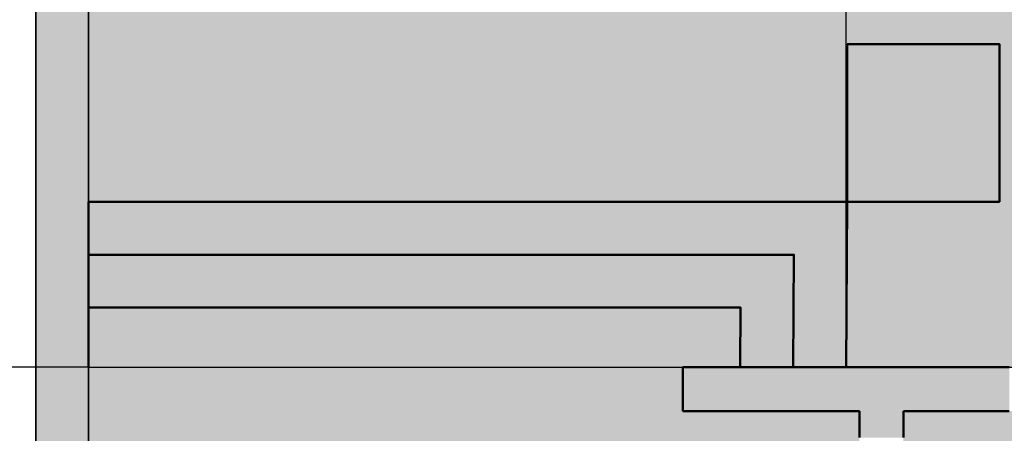
# Model space of a CAD drawing. Units: inches. Extents: x 925 to 2834, y 111 to 1355.
# Tile 15 of 25: x 1069 to 1293, y 1067 to 1160. Entities that reach past the tile are written whole.
import ezdxf

# ---------------------------------------------------------------- set-up
doc = ezdxf.new("R2010")
doc.units = ezdxf.units.IN
doc.header["$MEASUREMENT"] = 0
for name, color, linetype, lineweight in [('A-ANNO-DIMS', 2, 'Continuous', 18), ('A-ANNO-TTLB', 7, 'Continuous', 35), ('A-FLOR-PATT', 252, 'Continuous', 13), ('A-GLAZ', 3, 'Continuous', 25), ('A-WALL', 7, 'Continuous', 50)]:
    doc.layers.add(name, color=color, linetype=linetype, lineweight=lineweight)
doc.styles.get("Standard").update_dxf_attribs({"font": 'arial.ttf'})
doc.dimstyles.get("Standard").update_dxf_attribs({"dimtxt": 6, "dimasz": 3, "dimexe": 0.18, "dimexo": 0.0625, "dimgap": 0.09, "dimtad": 0, "dimtih": 1, "dimtoh": 1, "dimdec": 1, "dimzin": 0, "dimdsep": 46, "dimlunit": 3, "dimtxsty": 'Standard', "dimblk": 'ARCHTICK', "dimcen": 0.09, "dimadec": 0, "dimazin": 0, "dimtfac": 1, "dimtdec": 1, "dimtofl": 0, "dimtmove": 0, "dimatfit": 3, "dimfxl": 1, "dimtolj": 1, "dimtzin": 0, "dimarcsym": 0})

# ---------------------------------------------------------------- blocks, each defined once
blk = doc.blocks.new('_ArchTick')
at = {"color": 0, "linetype": 'ByBlock', "const_width": 0.15}
blk.add_lwpolyline([(-0.5, -0.5), (0.5, 0.5)], dxfattribs=at)
blk = doc.blocks.new('*D15')
at = {"layer": 'A-ANNO-DIMS', "color": 0, "lineweight": -2, "transparency": 16777216}
for p, q in [((1084.71, 1081.65), (1084.71, 1351.49)), ((1084.71, 1351.31), (1158.43, 1351.31)), ((1256.67, 1351.31), (1182.95, 1351.31)), ((1256.67, 1081.65), (1256.67, 1351.49))]:
    blk.add_line(p, q, dxfattribs=at)
at = {"layer": 'Defpoints', "color": 0, "transparency": 16777216}
for p in [(1256.67, 1351.31), (1084.71, 1081.59), (1256.67, 1081.59)]:
    blk.add_point(p, dxfattribs=at)
at = {"layer": 'A-ANNO-DIMS', "color": 0, "lineweight": -2, "transparency": 16777216, "xscale": 3, "yscale": 3, "zscale": 3, "rotation": 180}
blk.add_blockref('_ArchTick', (1084.71, 1351.31), dxfattribs=at)
at = {"layer": 'A-ANNO-DIMS', "color": 0, "lineweight": -2, "transparency": 16777216, "xscale": 3, "yscale": 3, "zscale": 3}
blk.add_blockref('_ArchTick', (1256.67, 1351.31), dxfattribs=at)
at = {"layer": 'A-ANNO-DIMS', "color": 0, "transparency": 16777216, "insert": (1170.69, 1351.31), "char_height": 6, "attachment_point": 5}
blk.add_mtext('\\A1;171.96', dxfattribs=at)
blk = doc.blocks.new('*D16')
at = {"layer": 'A-ANNO-DIMS', "color": 0, "lineweight": -2, "transparency": 16777216}
for p, q in [((1256.67, 1081.65), (1256.67, 1351.49)), ((1256.67, 1351.31), (1412.16, 1351.31)), ((1592.71, 1351.31), (1437.22, 1351.31)), ((1592.71, 1071.65), (1592.71, 1351.49))]:
    blk.add_line(p, q, dxfattribs=at)
at = {"layer": 'Defpoints', "color": 0, "transparency": 16777216}
for p in [(1592.71, 1351.31), (1256.67, 1081.59), (1592.71, 1071.59)]:
    blk.add_point(p, dxfattribs=at)
at = {"layer": 'A-ANNO-DIMS', "color": 0, "lineweight": -2, "transparency": 16777216, "xscale": 3, "yscale": 3, "zscale": 3, "rotation": 180}
blk.add_blockref('_ArchTick', (1256.67, 1351.31), dxfattribs=at)
at = {"layer": 'A-ANNO-DIMS', "color": 0, "lineweight": -2, "transparency": 16777216, "xscale": 3, "yscale": 3, "zscale": 3}
blk.add_blockref('_ArchTick', (1592.71, 1351.31), dxfattribs=at)
at = {"layer": 'A-ANNO-DIMS', "color": 0, "transparency": 16777216, "insert": (1424.69, 1351.31), "char_height": 6, "attachment_point": 5}
blk.add_mtext('\\A1;336.04', dxfattribs=at)
blk = doc.blocks.new('*D36')
at = {"layer": 'A-ANNO-DIMS', "color": 0, "lineweight": -2, "transparency": 16777216}
for p, q in [((1084.65, 1081.59), (934.81, 1081.59)), ((934.99, 1081.59), (934.99, 907.74)), ((934.99, 727.59), (934.99, 901.43)), ((1084.65, 727.59), (934.81, 727.59))]:
    blk.add_line(p, q, dxfattribs=at)
at = {"layer": 'Defpoints', "color": 0, "transparency": 16777216}
for p in [(934.99, 1081.59), (1084.71, 1081.59), (1084.71, 727.59)]:
    blk.add_point(p, dxfattribs=at)
at = {"layer": 'A-ANNO-DIMS', "color": 0, "lineweight": -2, "transparency": 16777216, "xscale": 3, "yscale": 3, "zscale": 3}
for p, rotation in [((934.99, 1081.59), 90), ((934.99, 727.59), 270)]:
    blk.add_blockref('_ArchTick', p, dxfattribs=dict(at, rotation=rotation))
at = {"layer": 'A-ANNO-DIMS', "color": 0, "transparency": 16777216, "insert": (934.99, 904.59), "char_height": 6, "attachment_point": 5}
blk.add_mtext('\\A1;354', dxfattribs=at)
blk = doc.blocks.new('*D37')
at = {"layer": 'A-ANNO-DIMS', "color": 0, "lineweight": -2, "transparency": 16777216}
for p, q in [((1084.65, 1201.59), (934.81, 1201.59)), ((934.99, 1201.59), (934.99, 1144.74)), ((934.99, 1081.59), (934.99, 1138.44)), ((1084.65, 1081.59), (934.81, 1081.59))]:
    blk.add_line(p, q, dxfattribs=at)
at = {"layer": 'Defpoints', "color": 0, "transparency": 16777216}
for p in [(934.99, 1201.59), (1084.71, 1201.59), (1084.71, 1081.59)]:
    blk.add_point(p, dxfattribs=at)
at = {"layer": 'A-ANNO-DIMS', "color": 0, "lineweight": -2, "transparency": 16777216, "xscale": 3, "yscale": 3, "zscale": 3}
for p, rotation in [((934.99, 1201.59), 90), ((934.99, 1081.59), 270)]:
    blk.add_blockref('_ArchTick', p, dxfattribs=dict(at, rotation=rotation))
at = {"layer": 'A-ANNO-DIMS', "color": 0, "transparency": 16777216, "insert": (934.99, 1141.59), "char_height": 6, "attachment_point": 5}
blk.add_mtext('\\A1;120', dxfattribs=at)

msp = doc.modelspace()

# ---------------------------------------------------------------- hatches: boundary and pattern name
at = {"layer": 'A-FLOR-PATT', "transparency": 33554605}
h = msp.add_hatch(color=256, dxfattribs=at)
h.dxf.hatch_style = 1
h.paths.add_polyline_path([(1931.688, 1294.5638), (991.7375, 1294.5638), (991.7375, 172.1134), (1931.688, 172.1134)])
h.paths.add_polyline_path([(1910.7128, 1273.5886), (1910.7128, 193.0886), (1012.7128, 193.0886), (1012.7128, 1273.5886)], flags=16)
h.paths.add_polyline_path([(1850.7128, 1213.5886), (1850.7128, 253.0886), (1072.7128, 253.0886), (1072.7128, 1213.5886)], flags=0)
h.paths.add_polyline_path([(1838.7128, 1201.5886), (1838.7128, 265.0886), (1084.7128, 265.0886), (1084.7128, 530.5886), (1084.7128, 1201.5886)], flags=0)
h.paths.add_polyline_path([(1547.6758, 1155.7396), (1547.6758, 1119.115), (1513.0687, 1119.115), (1513.0687, 1155.7396)], flags=0)
h.paths.add_polyline_path([(1600.1067, 1154.9439), (1634.7139, 1154.9439), (1634.7139, 1119.115), (1600.1067, 1119.115)], flags=0)
h.paths.add_polyline_path([(1505.2502, 1144.5358), (1505.2502, 1119.115), (1470.643, 1119.115), (1470.643, 1144.5358)], flags=0)
h.paths.add_polyline_path([(1559.1357, 1141.0962), (1593.7428, 1141.0962), (1593.7428, 1119.115), (1559.1357, 1119.115)], flags=0)
h.paths.add_polyline_path([(1462.8966, 1154.9439), (1462.8966, 1119.115), (1428.2895, 1119.115), (1428.2895, 1154.9439)], flags=0)
h.paths.add_polyline_path([(1642.4603, 1144.5358), (1677.0675, 1144.5358), (1677.0675, 1119.115), (1642.4603, 1119.115)], flags=0)
h.paths.add_polyline_path([(1422.3508, 1141.0962), (1422.3508, 1119.115), (1387.7436, 1119.115), (1387.7436, 1141.0962)], flags=0)
h.paths.add_polyline_path([(1684.8859, 1155.7396), (1719.4931, 1155.7396), (1719.4931, 1119.115), (1684.8859, 1119.115)], flags=0)
h.paths.add_polyline_path([(1718.7128, 1081.5886), (1718.7128, 1050.1249), (1715.7128, 1050.1249), (1715.7128, 1026.1249), (1715.7128, 1002.1249), (1718.7128, 1002.1249), (1730.7128, 1002.1249), (1730.7128, 998.1249), (1730.7128, 990.1249), (1730.7128, 986.1249), (1718.7128, 986.1249), (1718.7128, 893.5886), (1715.3735, 893.5886), (1715.3735, 891.5886), (1713.3735, 891.5886, 0.41421356), (1677.3735, 855.5886), (1713.3735, 855.5886), (1713.3735, 853.5886), (1715.3735, 853.5886), (1715.3735, 851.5886), (1718.7128, 851.5886), (1718.7128, 821.5865), (1734.4655, 821.5865), (1734.3735, 819.5886, -0.41421356), (1712.4415, 793.5886), (1712.4415, 791.5886), (1718.7128, 791.5886), (1718.7128, 717.5886), (1718.7128, 669.5886), (1732.7128, 669.5886), (1732.7128, 665.5886), (1732.7128, 641.5886), (1732.7128, 634.5886), (1732.7128, 610.5886), (1732.7128, 603.5886), (1718.7128, 603.5886), (1718.7128, 385.0886), (1434.2128, 385.0886), (1434.2128, 530.5886), (1410.2128, 530.5886), (1408.2128, 530.5886), (1408.2128, 532.5886, 0.41421356), (1372.2128, 568.5886), (1372.2128, 532.5886), (1370.2128, 532.5886), (1370.2128, 530.5886), (1368.2128, 530.5886), (1282.2128, 530.5886), (1210.2128, 530.5886), (1200.2128, 530.5886), (1200.2128, 542.1915), (1183.2307, 542.1915), (1183.2307, 546.1915), (1200.2128, 546.1915), (1200.2128, 572.1915), (1183.2307, 572.1915), (1183.2307, 576.1915), (1200.2128, 576.1915), (1200.2128, 727.5886), (1210.2128, 727.5886), (1234.2128, 727.5886), (1259.7128, 727.5886), (1259.7128, 775.5886), (1259.7128, 799.5886), (1259.7128, 847.5886), (1259.7128, 993.5872), (1259.7128, 1065.5872), (1259.7128, 1071.5886), (1219.6318, 1071.5886), (1219.6318, 1081.5886), (1084.7128, 1081.5886), (1084.7128, 1119.115), (1256.8974, 1119.115), (1256.8974, 1154.9439), (1291.5046, 1154.9439), (1291.5046, 1119.115), (1256.8974, 1119.115), (1256.6723, 1081.5886), (1293.7128, 1081.5886), (1341.7128, 1081.5886), (1341.7128, 1093.5886), (1347.7128, 1093.5886), (1371.7128, 1093.5886), (1377.7128, 1093.5886), (1377.7128, 1081.5886), (1668.7128, 1081.5886), (1668.7128, 1117.5886), (1675.7128, 1117.5886), (1711.7128, 1117.5886), (1718.7128, 1117.5886)], flags=0)
h.paths.add_polyline_path([(1376.2838, 1155.7396), (1376.2838, 1119.115), (1341.6766, 1119.115), (1341.6766, 1155.7396)], flags=0)
h.paths.add_polyline_path([(1341.7128, 1076.0886), (1293.7128, 1076.0886), (1293.7128, 1071.5886), (1269.7128, 1071.5886), (1269.7128, 1065.5872), (1266.7128, 1065.5872), (1266.7128, 1029.5872), (1265.7128, 1029.5872), (1265.7128, 993.5872), (1269.7128, 993.5872), (1269.7128, 903.5886), (1269.7128, 893.5886), (1269.7128, 847.5886), (1265.2128, 847.5886), (1265.2128, 799.5886), (1269.7128, 799.5886), (1269.7128, 775.5886), (1265.2128, 775.5886), (1265.2128, 727.5886), (1269.7128, 727.5886), (1444.2128, 727.5886), (1444.2128, 717.5886), (1234.2128, 717.5886), (1234.2128, 722.0886), (1210.2128, 722.0886), (1210.2128, 717.5886), (1210.2128, 540.5886), (1210.2128, 536.0886), (1282.2128, 536.0886), (1282.2128, 535.0886), (1210.2128, 535.0886), (1210.2128, 540.5886), (1210.2128, 717.5886), (1210.2128, 723.0886), (1234.2128, 723.0886), (1234.2128, 717.5886), (1444.2128, 717.5886), (1444.2128, 727.5886), (1269.7128, 727.5886), (1264.2128, 727.5886), (1264.2128, 775.5886), (1269.7128, 775.5886), (1269.7128, 799.5886), (1264.2128, 799.5886), (1264.2128, 847.5886), (1269.7128, 847.5886), (1269.7128, 893.5886), (1269.7128, 903.5886), (1269.7128, 993.5872), (1264.7128, 993.5872), (1264.7128, 1029.5872), (1265.7128, 1029.5872), (1265.7128, 1065.5872), (1269.7128, 1065.5872), (1269.7128, 1071.5886), (1293.7128, 1071.5886), (1293.7128, 1077.0886), (1341.7128, 1077.0886)], flags=0)
h.paths.add_polyline_path([(1730.9529, 1141.0962), (1765.5601, 1141.0962), (1765.5601, 1119.115), (1730.9529, 1119.115)], flags=0)
h.paths.add_polyline_path([(1333.8582, 1144.5358), (1333.8582, 1119.115), (1299.251, 1119.115), (1299.251, 1144.5358)], flags=0)
h.paths.add_polyline_path([(1592.7128, 968.5886), (1596.0342, 968.5886), (1602.7128, 968.5886), (1708.7128, 968.5886), (1708.7128, 903.5886), (1602.7128, 903.5886), (1602.7128, 938.5886), (1592.7128, 938.5886), (1592.7128, 903.5886), (1451.7128, 903.5886), (1451.7128, 893.5886), (1511.7128, 893.5886), (1511.7128, 881.5886), (1515.2128, 881.5886), (1518.7128, 881.5886), (1518.7128, 893.5886), (1592.7128, 893.5886), (1592.7128, 799.5886), (1518.7128, 799.5886), (1518.7128, 857.5886), (1511.7128, 857.5886), (1511.7128, 799.5886), (1511.7128, 772.0886), (1521.7128, 772.0886), (1521.7128, 792.5886), (1592.7128, 792.5886), (1592.7128, 727.5886), (1521.7128, 727.5886), (1521.7128, 748.0886), (1511.7128, 748.0886), (1511.7128, 717.5886), (1708.7128, 717.5886), (1714.2128, 717.5886), (1714.2128, 669.5886), (1708.7128, 669.5886), (1708.7128, 641.5886), (1492.2128, 641.5886), (1492.2128, 631.5886), (1621.2128, 631.5886), (1621.2128, 443.0886), (1625.7128, 443.0886), (1625.7128, 503.0886), (1625.7128, 507.5886), (1625.7128, 631.5886), (1708.7128, 631.5886), (1708.7128, 507.5886), (1655.7128, 507.5886), (1655.7128, 503.0886), (1708.7128, 503.0886), (1708.7128, 395.0886), (1625.7128, 395.0886), (1625.7128, 419.0886), (1621.2128, 419.0886), (1621.2128, 395.0886), (1482.2128, 395.0886), (1482.2128, 385.0886), (1434.2128, 385.0886), (1434.2128, 433.0886), (1444.2128, 433.0886), (1444.2128, 631.5886), (1450.2128, 631.5886), (1450.2128, 634.91), (1452.2128, 634.91), (1452.2128, 669.5886), (1454.2128, 669.5886, -0.40021217), (1490.1712, 635.3173), (1492.2128, 635.3173), (1492.2128, 641.5886), (1564.7128, 641.5886), (1564.7128, 677.5886), (1672.7128, 677.5886), (1672.7128, 681.5886), (1564.7128, 681.5886), (1564.7128, 717.5886), (1511.7128, 717.5886), (1511.7128, 748.0886), (1511.7128, 772.0886), (1511.7128, 799.5886), (1511.7128, 857.5886), (1511.8913, 857.5886), (1511.8913, 859.5886), (1515.6201, 859.5886, 0.41421356), (1537.552, 879.5886), (1513.552, 879.5886), (1511.8913, 879.5886), (1511.8913, 881.5886), (1511.7128, 881.5886), (1511.7128, 893.5886), (1451.7128, 893.5886), (1451.7128, 903.5886), (1592.7128, 903.5886), (1592.7128, 938.5886), (1592.7128, 940.5886), (1596.4415, 940.5886, 0.41421356), (1618.3735, 966.5886), (1594.3735, 966.5886), (1592.7128, 966.5886)], flags=0)
h.paths.add_polyline_path([(1377.7128, 903.5886), (1377.7128, 893.5886), (1305.7128, 893.5886), (1305.7128, 903.5886)], flags=0)
h.paths.add_polyline_path([(1708.7128, 821.5886), (1712.0342, 821.5886), (1712.0342, 819.5886), (1710.3735, 819.5886), (1708.7128, 819.5886)], flags=0)
h.paths.add_polyline_path([(1576.7128, 695.1992), (1575.5896, 693.6649), (1575.9687, 694.6994), (1575.4438, 695.1992), (1575.9687, 695.699), (1575.5896, 696.7335)], flags=0)
h.paths.add_polyline_path([(1565.9817, 662.3134), (1565.4568, 661.8136), (1565.8359, 660.7791), (1564.7128, 662.3134), (1565.8359, 663.8477), (1565.4568, 662.8132)], flags=0)
h.paths.add_polyline_path([(1444.2128, 433.0886), (1444.2128, 395.0886), (1482.2128, 395.0886), (1482.2128, 389.0886), (1438.2128, 389.0886), (1438.2128, 391.8608), (1438.2128, 433.0886)], flags=0)
h.paths.add_polyline_path([(1410.2128, 506.5886), (1410.2128, 289.0886), (1108.7128, 289.0886), (1108.7128, 506.5886)], flags=0)
h.paths.add_polyline_path([(1612.3153, 838.3016), (1680.4151, 838.3016), (1680.4151, 851.3131), (1612.3153, 851.3131)], flags=8)
h.paths.add_polyline_path([(1208.3174, 395.0436), (1282.1017, 395.0436), (1282.1017, 408.0552), (1208.3174, 408.0552)], flags=8)
h.paths.add_polyline_path([(1291.8049, 598.7427), (1369.8017, 598.7427), (1369.8017, 611.7542), (1291.8049, 611.7542)], flags=8)
h.paths.add_polyline_path([(1119.679, 917.3022), (1191.0817, 917.3022), (1191.0817, 930.3137), (1119.679, 930.3137)], flags=8)
h.paths.add_polyline_path([(1332.2261, 815.9808), (1410.2258, 815.9808), (1410.2258, 829.001), (1332.2261, 829.001)], flags=8)
h.paths.add_polyline_path([(1390.9013, 955.8158), (1475.4981, 955.8158), (1475.4981, 968.8273), (1390.9013, 968.8273)], flags=8)
h.paths.add_polyline_path([(1620.3436, 998.9325), (1688.4434, 998.9325), (1688.4434, 1011.944), (1620.3436, 1011.944)], flags=8)
h.paths.add_polyline_path([(1620.3436, 914.1039), (1691.7405, 914.1039), (1691.7405, 927.1155), (1620.3436, 927.1155)], flags=8)
h.paths.add_polyline_path([(1521.4542, 816.005), (1589.5569, 816.005), (1589.5569, 829.0253), (1521.4542, 829.0253)], flags=8)
h.paths.add_polyline_path([(1528.524, 740.3497), (1602.3082, 740.3497), (1602.3082, 753.3613), (1528.524, 753.3613)], flags=8)
h.paths.add_polyline_path([(1627.6094, 762.6128), (1702.3091, 762.6128), (1702.3091, 775.6244), (1627.6094, 775.6244)], flags=8)
h.paths.add_polyline_path([(1610.5442, 657.2751), (1684.3284, 657.2751), (1684.3284, 670.2867), (1610.5442, 670.2867)], flags=8)
h.paths.add_polyline_path([(1636.6983, 519.472), (1711.3981, 519.472), (1711.3981, 532.4835), (1636.6983, 532.4835)], flags=8)
h.paths.add_polyline_path([(1616.8577, 424.8539), (1694.8545, 424.8539), (1694.8545, 437.8654), (1616.8577, 437.8654)], flags=8)
h.paths.add_polyline_path([(1506.1456, 460.8838), (1579.9299, 460.8838), (1579.9299, 473.8953), (1506.1456, 473.8953)], flags=8)
h.paths.add_polyline_path([(1624.6119, 784.6011), (1696.9185, 784.6011), (1696.9185, 797.7864), (1624.6119, 797.7864)], flags=8)
h.paths.add_polyline_path([(1606.3732, 854.2194), (1683.3039, 854.2194), (1683.3039, 867.4048), (1606.3732, 867.4048)], flags=8)
h.paths.add_polyline_path([(1127.8008, 940.3581), (1165.1637, 940.3581), (1165.1637, 953.5348), (1127.8008, 953.5348)], flags=8)
h.paths.add_polyline_path([(1620.8657, 1019.4968), (1677.3447, 1019.4968), (1677.3447, 1032.6735), (1620.8657, 1032.6735)], flags=8)
h.paths.add_polyline_path([(1620.8643, 930.1821), (1703.0564, 930.1821), (1703.0564, 943.3675), (1620.8643, 943.3675)], flags=8)
h.paths.add_polyline_path([(1324.5702, 836.8338), (1408.0892, 836.8338), (1408.0892, 850.0191), (1324.5702, 850.0191)], flags=8)
h.paths.add_polyline_path([(1281.6584, 622.8885), (1383.6213, 622.8885), (1383.6213, 636.0739), (1281.6584, 636.0739)], flags=8)
h.paths.add_polyline_path([(1210.6721, 416.7893), (1269.1299, 416.7893), (1269.1299, 429.9747), (1210.6721, 429.9747)], flags=8)
h.paths.add_polyline_path([(1507.8264, 477.4836), (1586.7329, 477.4836), (1586.7329, 490.669), (1507.8264, 490.669)], flags=8)
h.paths.add_polyline_path([(1643.6238, 443.8135), (1696.6696, 443.8135), (1696.6696, 456.5643), (1643.6238, 456.5643)], flags=8)
h.paths.add_polyline_path([(1647.2466, 540.5638), (1693.1825, 540.5638), (1693.1825, 553.7491), (1647.2466, 553.7491)], flags=8)
h.paths.add_polyline_path([(1626.0633, 668.5064), (1673.3174, 668.5064), (1673.3174, 681.6831), (1626.0633, 681.6831)], flags=8)
h.paths.add_polyline_path([(1538.2915, 830.7872), (1567.5942, 830.7872), (1567.5942, 843.5293), (1538.2915, 843.5293)], flags=8)
h.paths.add_polyline_path([(1530.9338, 754.0477), (1559.576, 754.0477), (1559.576, 766.7898), (1530.9338, 766.7898)], flags=8)
h.paths.add_polyline_path([(1351.2461, 979.2309), (1513.8919, 979.2309), (1513.8919, 992.4076), (1351.2461, 992.4076)], flags=8)
at = {"layer": 'A-FLOR-PATT'}
h = msp.add_hatch(color=256, dxfattribs=at)
h.dxf.hatch_style = 1
h.paths.add_polyline_path([(1850.7128, 1213.5886), (1072.7128, 1213.5886), (1072.7128, 253.0886), (1850.7128, 253.0886)])
h.paths.add_polyline_path([(1084.7128, 1201.5886), (1838.7128, 1201.5886), (1838.7128, 265.0886), (1084.7128, 265.0886)], flags=16)
h.paths.add_polyline_path([(1183.2307, 576.1915), (1200.2128, 576.1915), (1200.2128, 727.5886), (1210.2128, 727.5886), (1234.2128, 727.5886), (1259.7128, 727.5886), (1259.7128, 775.5886), (1259.7128, 799.5886), (1259.7128, 847.5886), (1259.7128, 993.5872), (1259.7128, 1065.5872), (1259.7128, 1071.5886), (1219.6318, 1071.5886), (1219.6318, 1081.5886), (1293.7128, 1081.5886), (1341.7128, 1081.5886), (1341.7128, 1093.5886), (1347.7128, 1093.5886), (1347.7128, 1081.5886), (1371.7128, 1081.5886), (1371.7128, 1093.5886), (1377.7128, 1093.5886), (1377.7128, 1081.5886), (1668.7128, 1081.5886), (1668.7128, 1117.5886), (1675.7128, 1117.5886), (1675.7128, 1081.5886), (1711.7128, 1081.5886), (1711.7128, 1117.5886), (1718.7128, 1117.5886), (1718.7128, 1081.5886), (1718.7128, 1050.1249), (1715.7128, 1050.1249), (1715.7128, 1026.1249), (1715.7128, 1002.1249), (1718.7128, 1002.1249), (1730.7128, 1002.1249), (1730.7128, 998.1249), (1730.7128, 990.1249), (1730.7128, 986.1249), (1718.7128, 986.1249), (1718.7128, 893.5886), (1715.3735, 893.5886), (1715.3735, 891.5886), (1713.3735, 891.5886, 0.41421356), (1677.3735, 855.5886), (1713.3735, 855.5886), (1713.3735, 853.5886), (1715.3735, 853.5886), (1715.3735, 851.5886), (1718.7128, 851.5886), (1718.7128, 821.5865), (1734.4655, 821.5865), (1734.3735, 819.5886, -0.41421356), (1712.4415, 793.5886), (1712.4415, 791.5886), (1718.7128, 791.5886), (1718.7128, 717.5886), (1718.7128, 669.5886), (1732.7128, 669.5886), (1732.7128, 665.5886), (1732.7128, 641.5886), (1732.7128, 634.5886), (1732.7128, 610.5886), (1732.7128, 603.5886), (1718.7128, 603.5886), (1718.7128, 385.0886), (1434.2128, 385.0886), (1434.2128, 433.0886), (1434.2128, 530.5886), (1410.2128, 530.5886), (1408.2128, 530.5886), (1408.2128, 532.5886, 0.41421356), (1372.2128, 568.5886), (1372.2128, 532.5886), (1370.2128, 532.5886), (1370.2128, 530.5886), (1368.2128, 530.5886), (1282.2128, 530.5886), (1210.2128, 530.5886), (1200.2128, 530.5886), (1200.2128, 542.1915), (1183.2307, 542.1915), (1183.2307, 546.1915), (1200.2128, 546.1915), (1200.2128, 572.1915), (1183.2307, 572.1915)], flags=0)
h.paths.add_polyline_path([(1210.2128, 717.5886), (1210.2128, 723.0886), (1234.2128, 723.0886), (1234.2128, 717.5886), (1444.2128, 717.5886), (1444.2128, 727.5886), (1269.7128, 727.5886), (1264.2128, 727.5886), (1264.2128, 775.5886), (1269.7128, 775.5886), (1269.7128, 799.5886), (1264.2128, 799.5886), (1264.2128, 847.5886), (1269.7128, 847.5886), (1269.7128, 893.5886), (1269.7128, 903.5886), (1269.7128, 993.5872), (1264.7128, 993.5872), (1264.7128, 1029.5872), (1265.7128, 1029.5872), (1265.7128, 1065.5872), (1269.7128, 1065.5872), (1269.7128, 1071.5886), (1293.7128, 1071.5886), (1293.7128, 1077.0886), (1341.7128, 1077.0886), (1341.7128, 1076.0886), (1293.7128, 1076.0886), (1293.7128, 1071.5886), (1269.7128, 1071.5886), (1269.7128, 1065.5872), (1266.7128, 1065.5872), (1266.7128, 1029.5872), (1265.7128, 1029.5872), (1265.7128, 993.5872), (1269.7128, 993.5872), (1269.7128, 903.5886), (1269.7128, 893.5886), (1269.7128, 847.5886), (1265.2128, 847.5886), (1265.2128, 799.5886), (1269.7128, 799.5886), (1269.7128, 775.5886), (1265.2128, 775.5886), (1265.2128, 727.5886), (1269.7128, 727.5886), (1444.2128, 727.5886), (1444.2128, 717.5886), (1234.2128, 717.5886), (1234.2128, 722.0886), (1210.2128, 722.0886), (1210.2128, 717.5886), (1210.2128, 540.5886), (1210.2128, 536.0886), (1282.2128, 536.0886), (1282.2128, 535.0886), (1210.2128, 535.0886), (1210.2128, 540.5886)], flags=0)
h.paths.add_polyline_path([(1450.2128, 634.91), (1452.2128, 634.91), (1452.2128, 669.5886), (1454.2128, 669.5886, -0.40021217), (1490.1712, 635.3173), (1492.2128, 635.3173), (1492.2128, 641.5886), (1564.7128, 641.5886), (1564.7128, 677.5886), (1672.7128, 677.5886), (1672.7128, 681.5886), (1564.7128, 681.5886), (1564.7128, 717.5886), (1511.7128, 717.5886), (1511.7128, 748.0886), (1511.7128, 772.0886), (1511.7128, 799.5886), (1511.7128, 857.5886), (1511.8913, 857.5886), (1511.8913, 859.5886), (1515.6201, 859.5886, 0.41421356), (1537.552, 879.5886), (1513.552, 879.5886), (1511.8913, 879.5886), (1511.8913, 881.5886), (1511.7128, 881.5886), (1511.7128, 893.5886), (1451.7128, 893.5886), (1451.7128, 903.5886), (1592.7128, 903.5886), (1592.7128, 938.5886), (1592.7128, 940.5886), (1596.4415, 940.5886, 0.41421356), (1618.3735, 966.5886), (1594.3735, 966.5886), (1592.7128, 966.5886), (1592.7128, 968.5886), (1596.0342, 968.5886), (1602.7128, 968.5886), (1708.7128, 968.5886), (1708.7128, 903.5886), (1602.7128, 903.5886), (1602.7128, 938.5886), (1592.7128, 938.5886), (1592.7128, 903.5886), (1451.7128, 903.5886), (1451.7128, 893.5886), (1511.7128, 893.5886), (1511.7128, 881.5886), (1518.7128, 881.5886), (1518.7128, 893.5886), (1592.7128, 893.5886), (1592.7128, 799.5886), (1518.7128, 799.5886), (1518.7128, 857.5886), (1511.7128, 857.5886), (1511.7128, 799.5886), (1511.7128, 772.0886), (1521.7128, 772.0886), (1521.7128, 792.5886), (1592.7128, 792.5886), (1592.7128, 727.5886), (1521.7128, 727.5886), (1521.7128, 748.0886), (1511.7128, 748.0886), (1511.7128, 717.5886), (1708.7128, 717.5886), (1714.2128, 717.5886), (1714.2128, 669.5886), (1708.7128, 669.5886), (1708.7128, 641.5886), (1492.2128, 641.5886), (1492.2128, 631.5886), (1621.2128, 631.5886), (1621.2128, 443.0886), (1625.7128, 443.0886), (1625.7128, 503.0886), (1625.7128, 507.5886), (1625.7128, 631.5886), (1708.7128, 631.5886), (1708.7128, 507.5886), (1655.7128, 507.5886), (1655.7128, 503.0886), (1708.7128, 503.0886), (1708.7128, 395.0886), (1625.7128, 395.0886), (1625.7128, 419.0886), (1621.2128, 419.0886), (1621.2128, 395.0886), (1482.2128, 395.0886), (1482.2128, 389.0886), (1438.2128, 389.0886), (1438.2128, 391.8608), (1438.2128, 433.0886), (1444.2128, 433.0886), (1444.2128, 631.5886), (1450.2128, 631.5886)], flags=0)
h.paths.add_polyline_path([(1444.2128, 433.0886), (1444.2128, 395.0886), (1482.2128, 395.0886), (1482.2128, 391.0886), (1440.2128, 391.0886), (1440.2128, 391.8608), (1440.2128, 433.0886)], flags=0)
h.paths.add_polyline_path([(1305.7128, 893.5886), (1305.7128, 903.5886), (1377.7128, 903.5886), (1377.7128, 893.5886)], flags=0)
h.paths.add_polyline_path([(1564.7128, 662.3134), (1565.8359, 663.8477), (1565.4568, 662.8132), (1565.9817, 662.3134), (1565.4568, 661.8136), (1565.8359, 660.7791)], flags=0)
h.paths.add_polyline_path([(1575.4438, 695.1992), (1575.9687, 695.699), (1575.5896, 696.7335), (1576.7128, 695.1992), (1575.5896, 693.6649), (1575.9687, 694.6994)], flags=0)
h.paths.add_polyline_path([(1708.7128, 821.5886), (1712.0342, 821.5886), (1712.0342, 819.5886), (1710.3735, 819.5886), (1708.7128, 819.5886)], flags=0)
at = {"layer": 'A-FLOR-PATT', "transparency": 33554554}
h = msp.add_hatch(color=256, dxfattribs=at)
h.dxf.hatch_style = 1
h.paths.add_polyline_path([(1838.7128, 1201.5886), (1084.7128, 1201.5886), (1084.7128, 1119.115), (1256.8974, 1119.115), (1256.8974, 1154.9439), (1291.5046, 1154.9439), (1291.5046, 1119.115), (1256.8974, 1119.115), (1256.6723, 1081.5886), (1293.7128, 1081.5886), (1341.7128, 1081.5886), (1341.7128, 1093.5886), (1347.7128, 1093.5886), (1371.7128, 1093.5886), (1377.7128, 1093.5886), (1377.7128, 1081.5886), (1668.7128, 1081.5886), (1668.7128, 1117.5886), (1675.7128, 1117.5886), (1711.7128, 1117.5886), (1718.7128, 1117.5886), (1718.7128, 1081.5886), (1838.7128, 1081.5886)])
h.paths.add_polyline_path([(1299.251, 1144.5358), (1333.8582, 1144.5358), (1333.8582, 1119.115), (1299.251, 1119.115)], flags=16)
h.paths.add_polyline_path([(1341.6766, 1155.7396), (1376.2838, 1155.7396), (1376.2838, 1119.115), (1341.6766, 1119.115)], flags=16)
h.paths.add_polyline_path([(1387.7436, 1141.0962), (1422.3508, 1141.0962), (1422.3508, 1119.115), (1387.7436, 1119.115)], flags=16)
h.paths.add_polyline_path([(1428.2895, 1154.9439), (1462.8966, 1154.9439), (1462.8966, 1119.115), (1428.2895, 1119.115)], flags=16)
h.paths.add_polyline_path([(1470.643, 1144.5358), (1505.2502, 1144.5358), (1505.2502, 1119.115), (1470.643, 1119.115)], flags=16)
h.paths.add_polyline_path([(1513.0687, 1155.7396), (1547.6758, 1155.7396), (1547.6758, 1119.115), (1513.0687, 1119.115)], flags=16)
h.paths.add_polyline_path([(1559.1357, 1141.0962), (1593.7428, 1141.0962), (1593.7428, 1119.115), (1559.1357, 1119.115)], flags=16)
h.paths.add_polyline_path([(1600.1067, 1154.9439), (1634.7139, 1154.9439), (1634.7139, 1119.115), (1600.1067, 1119.115)], flags=16)
h.paths.add_polyline_path([(1642.4603, 1144.5358), (1677.0675, 1144.5358), (1677.0675, 1119.115), (1642.4603, 1119.115)], flags=16)
h.paths.add_polyline_path([(1684.8859, 1155.7396), (1719.4931, 1155.7396), (1719.4931, 1119.115), (1684.8859, 1119.115)], flags=16)
h.paths.add_polyline_path([(1730.9529, 1141.0962), (1765.5601, 1141.0962), (1765.5601, 1119.115), (1730.9529, 1119.115)], flags=16)
at = {"layer": 'A-FLOR-PATT', "transparency": 33554661}
h = msp.add_hatch(color=256, dxfattribs=at)
h.dxf.hatch_style = 1
h.paths.add_polyline_path([(1291.5046, 1154.9439), (1256.8974, 1154.9439), (1256.8974, 1119.115), (1291.5046, 1119.115)])
h.paths.add_polyline_path([(1333.8582, 1144.5358), (1299.251, 1144.5358), (1299.251, 1119.115), (1333.8582, 1119.115)])
h.paths.add_polyline_path([(1376.2838, 1155.7396), (1341.6766, 1155.7396), (1341.6766, 1119.115), (1376.2838, 1119.115)])
h.paths.add_polyline_path([(1422.3508, 1141.0962), (1387.7436, 1141.0962), (1387.7436, 1119.115), (1422.3508, 1119.115)])
h.paths.add_polyline_path([(1462.8966, 1154.9439), (1428.2895, 1154.9439), (1428.2895, 1119.115), (1462.8966, 1119.115)])
h.paths.add_polyline_path([(1505.2502, 1144.5358), (1470.643, 1144.5358), (1470.643, 1119.115), (1505.2502, 1119.115)])
h.paths.add_polyline_path([(1547.6758, 1155.7396), (1513.0687, 1155.7396), (1513.0687, 1119.115), (1547.6758, 1119.115)])
h.paths.add_polyline_path([(1593.7428, 1141.0962), (1559.1357, 1141.0962), (1559.1357, 1119.115), (1593.7428, 1119.115)])
h.paths.add_polyline_path([(1634.7139, 1154.9439), (1600.1067, 1154.9439), (1600.1067, 1119.115), (1634.7139, 1119.115)])
h.paths.add_polyline_path([(1677.0675, 1144.5358), (1642.4603, 1144.5358), (1642.4603, 1119.115), (1677.0675, 1119.115)])
h.paths.add_polyline_path([(1719.4931, 1155.7396), (1684.8859, 1155.7396), (1684.8859, 1119.115), (1719.4931, 1119.115)])
h.paths.add_polyline_path([(1765.5601, 1141.0962), (1730.9529, 1141.0962), (1730.9529, 1119.115), (1765.5601, 1119.115)])
at = {"layer": 'A-FLOR-PATT', "transparency": 33554605}
h = msp.add_hatch(color=256, dxfattribs=at)
h.dxf.hatch_style = 1
h.paths.add_polyline_path([(1256.8974, 1119.115), (1084.7128, 1119.115), (1084.7128, 1107.115), (1244.8252, 1107.115), (1244.672, 1081.5886), (1256.6723, 1081.5886)])
h.paths.add_polyline_path([(1244.8252, 1107.115), (1084.7128, 1107.115), (1084.7128, 1095.115), (1232.753, 1095.115), (1232.6718, 1081.5886), (1244.672, 1081.5886)], flags=17)
h.paths.add_polyline_path([(1232.753, 1095.115), (1084.7128, 1095.115), (1084.7128, 1081.5886), (1232.6718, 1081.5886)], flags=16)
at = {"layer": 'A-FLOR-PATT'}
h = msp.add_hatch(color=256, dxfattribs=at)
h.dxf.hatch_style = 1
h.paths.add_polyline_path([(1718.7128, 603.5886), (1708.7128, 603.5886), (1708.7128, 507.5886), (1655.7128, 507.5886), (1655.7128, 503.0886), (1708.7128, 503.0886), (1708.7128, 395.0886), (1625.7128, 395.0886), (1625.7128, 419.0886), (1621.2128, 419.0886), (1621.2128, 395.0886), (1482.2128, 395.0886), (1482.2128, 385.0886), (1718.7128, 385.0886)])
h.paths.add_polyline_path([(1625.7128, 631.5886), (1708.7128, 631.5886), (1708.7128, 603.5886), (1718.7128, 603.5886), (1732.7128, 603.5886), (1732.7128, 610.5886), (1715.7128, 610.5886), (1715.7128, 634.5886), (1732.7128, 634.5886), (1732.7128, 641.5886), (1715.7128, 641.5886), (1715.7128, 665.5886), (1732.7128, 665.5886), (1732.7128, 669.5886), (1708.7128, 669.5886), (1708.7128, 641.5886), (1492.2128, 641.5886), (1492.2128, 631.5886), (1621.2128, 631.5886), (1621.2128, 443.0886), (1625.7128, 443.0886), (1625.7128, 503.0886), (1625.7128, 507.5886)])
h.paths.add_polyline_path([(1718.7128, 851.5886), (1708.7128, 851.5886), (1708.7128, 828.5886), (1602.7128, 828.5886), (1602.7128, 893.5886), (1708.7128, 893.5886), (1718.7128, 893.5886), (1718.7128, 986.1249), (1730.7128, 986.1249), (1730.7128, 990.1249), (1718.7128, 990.1249), (1718.7128, 998.1249), (1730.7128, 998.1249), (1730.7128, 1002.1249), (1718.7128, 1002.1249), (1708.7128, 1002.1249), (1708.7128, 975.5886), (1602.7128, 975.5886), (1602.7128, 1011.5886), (1592.7128, 1011.5886), (1592.7128, 968.5886), (1596.0342, 968.5886), (1602.7128, 968.5886), (1708.7128, 968.5886), (1708.7128, 903.5886), (1602.7128, 903.5886), (1602.7128, 938.5886), (1592.7128, 938.5886), (1592.7128, 903.5886), (1451.7128, 903.5886), (1451.7128, 893.5886), (1511.7128, 893.5886), (1511.7128, 881.5886), (1515.2128, 881.5886), (1518.7128, 881.5886), (1518.7128, 893.5886), (1592.7128, 893.5886), (1592.7128, 799.5886), (1518.7128, 799.5886), (1518.7128, 857.5886), (1511.7128, 857.5886), (1511.7128, 799.5886), (1511.7128, 772.0886), (1521.7128, 772.0886), (1521.7128, 792.5886), (1592.7128, 792.5886), (1592.7128, 727.5886), (1521.7128, 727.5886), (1521.7128, 748.0886), (1511.7128, 748.0886), (1511.7128, 717.5886), (1708.7128, 717.5886), (1718.7128, 717.5886), (1718.7128, 727.5886), (1718.7128, 791.5886), (1708.7128, 791.5886), (1708.7128, 727.5886), (1602.7128, 727.5886), (1602.7128, 821.5886), (1708.7128, 821.5886), (1712.0342, 821.5886), (1718.7128, 821.5886)])
h.paths.add_polyline_path([(1718.7128, 1081.5886), (1718.7128, 1117.5886), (1711.7128, 1117.5886), (1711.7128, 1081.5886), (1675.7128, 1081.5886), (1675.7128, 1117.5886), (1668.7128, 1117.5886), (1668.7128, 1081.5886), (1377.7128, 1081.5886), (1377.7128, 1093.5886), (1371.7128, 1093.5886), (1371.7128, 1081.5886), (1347.7128, 1081.5886), (1347.7128, 1093.5886), (1341.7128, 1093.5886), (1341.7128, 1081.5886), (1341.7128, 1071.5886), (1592.7128, 1071.5886), (1592.7128, 1035.5886), (1602.7128, 1035.5886), (1602.7128, 1071.5886), (1708.7128, 1071.5886), (1708.7128, 1050.1249), (1718.7128, 1050.1249)])
h.paths.add_polyline_path([(1293.7128, 1081.5886), (1219.6318, 1081.5886), (1219.6318, 1071.5886), (1259.7128, 1071.5886), (1259.7128, 1065.5872), (1269.7128, 1065.5872), (1269.7128, 1071.5886), (1293.7128, 1071.5886)])
h.paths.add_polyline_path([(1269.7128, 903.5886), (1269.7128, 993.5872), (1259.7128, 993.5872), (1259.7128, 847.5886), (1269.7128, 847.5886), (1269.7128, 893.5886)])
h.paths.add_polyline_path([(1377.7128, 903.5886), (1305.7128, 903.5886), (1305.7128, 893.5886), (1377.7128, 893.5886)])
h.paths.add_polyline_path([(1444.2128, 727.5886), (1269.7128, 727.5886), (1259.7128, 727.5886), (1234.2128, 727.5886), (1234.2128, 717.5886), (1444.2128, 717.5886)])
h.paths.add_polyline_path([(1269.7128, 799.5886), (1259.7128, 799.5886), (1259.7128, 775.5886), (1269.7128, 775.5886)])
h.paths.add_polyline_path([(1444.2128, 631.5886), (1450.2128, 631.5886), (1450.2128, 634.91), (1450.2128, 641.5886), (1434.2128, 641.5886), (1434.2128, 540.5886), (1410.2128, 540.5886), (1410.2128, 530.5886), (1434.2128, 530.5886), (1434.2128, 433.0886), (1444.2128, 433.0886)])
h.paths.add_polyline_path([(1368.2128, 533.91), (1368.2128, 540.5886), (1282.2128, 540.5886), (1282.2128, 530.5886), (1368.2128, 530.5886)])
h.paths.add_polyline_path([(1210.2128, 717.5886), (1210.2128, 727.5886), (1200.2128, 727.5886), (1200.2128, 576.1915), (1183.2307, 576.1915), (1183.2307, 572.1915), (1200.2128, 572.1915), (1200.2128, 546.1915), (1183.2307, 546.1915), (1183.2307, 542.1915), (1200.2128, 542.1915), (1200.2128, 530.5886), (1210.2128, 530.5886), (1210.2128, 540.5886)])
at = {"layer": 'A-FLOR-PATT', "transparency": 33554574}
h = msp.add_hatch(color=256, dxfattribs=at)
h.dxf.hatch_style = 1
h.paths.add_polyline_path([(1259.7128, 993.5872), (1259.7128, 1065.5872), (1259.7128, 1071.5886), (1219.6318, 1071.5886), (1219.6318, 1081.5886), (1084.7128, 1081.5886), (1084.7128, 727.5886), (1200.2128, 727.5886), (1210.2128, 727.5886), (1234.2128, 727.5886), (1259.7128, 727.5886), (1259.7128, 775.5886), (1259.7128, 799.5886), (1259.7128, 847.5886)])
at = {"layer": 'A-FLOR-PATT', "transparency": 33554605}
h = msp.add_hatch(color=256, dxfattribs=at)
h.dxf.hatch_style = 1
h.paths.add_polyline_path([(1592.7128, 938.5886), (1592.7128, 940.5886), (1596.4415, 940.5886, 0.41421356), (1618.3735, 966.5886), (1594.3735, 966.5886), (1592.7128, 966.5886), (1592.7128, 968.5886), (1592.7128, 1011.5886), (1602.7128, 1011.5886), (1602.7128, 975.5886), (1708.7128, 975.5886), (1708.7128, 1002.1249), (1711.7128, 1002.1249), (1711.7128, 1026.1249), (1711.7128, 1050.1249), (1708.7128, 1050.1249), (1708.7128, 1071.5886), (1602.7128, 1071.5886), (1602.7128, 1035.5886), (1592.7128, 1035.5886), (1592.7128, 1071.5886), (1341.7128, 1071.5886), (1293.7128, 1071.5886), (1269.7128, 1071.5886), (1269.7128, 1065.5872), (1269.7128, 993.5872), (1269.7128, 903.5886), (1269.7128, 893.5886), (1269.7128, 847.5886), (1269.7128, 799.5886), (1269.7128, 775.5886), (1269.7128, 727.5886), (1444.2128, 727.5886), (1444.2128, 717.5886), (1234.2128, 717.5886), (1210.2128, 717.5886), (1210.2128, 540.5886), (1282.2128, 540.5886), (1368.2128, 540.5886), (1368.2128, 533.91), (1370.2128, 533.91), (1370.2128, 568.5886), (1372.2128, 568.5886, -0.40021217), (1408.1712, 534.3173), (1410.2128, 534.3173), (1410.2128, 540.5886), (1434.2128, 540.5886), (1434.2128, 641.5886), (1450.2128, 641.5886), (1450.2128, 634.91), (1452.2128, 634.91), (1452.2128, 669.5886), (1454.2128, 669.5886, -0.40021217), (1490.1712, 635.3173), (1492.2128, 635.3173), (1492.2128, 641.5886), (1564.7128, 641.5886), (1564.7128, 677.5886), (1672.7128, 677.5886), (1672.7128, 681.5886), (1564.7128, 681.5886), (1564.7128, 717.5886), (1511.7128, 717.5886), (1511.7128, 748.0886), (1511.7128, 772.0886), (1511.7128, 799.5886), (1511.7128, 857.5886), (1511.8913, 857.5886), (1511.8913, 859.5886), (1515.6201, 859.5886, 0.41421356), (1537.552, 879.5886), (1513.552, 879.5886), (1511.8913, 879.5886), (1511.8913, 881.5886), (1511.7128, 881.5886), (1511.7128, 893.5886), (1451.7128, 893.5886), (1451.7128, 903.5886), (1592.7128, 903.5886)])
h.paths.add_polyline_path([(1377.7128, 903.5886), (1377.7128, 893.5886), (1305.7128, 893.5886), (1305.7128, 903.5886)], flags=16)
h.paths.add_polyline_path([(1592.7128, 893.5886), (1518.7128, 893.5886), (1518.7128, 881.5865), (1537.6441, 881.5865), (1537.552, 879.5886, -0.41421356), (1515.6201, 859.5886), (1515.6201, 857.5886), (1518.7128, 857.5886), (1518.7128, 799.5886), (1592.7128, 799.5886)], flags=17)
h.paths.add_polyline_path([(1291.8049, 598.7427), (1369.8017, 598.7427), (1369.8017, 611.7542), (1291.8049, 611.7542)], flags=24)
h.paths.add_polyline_path([(1332.2261, 815.9808), (1410.2258, 815.9808), (1410.2258, 829.001), (1332.2261, 829.001)], flags=24)
h.paths.add_polyline_path([(1390.9013, 955.8158), (1475.4981, 955.8158), (1475.4981, 968.8273), (1390.9013, 968.8273)], flags=24)
h.paths.add_polyline_path([(1620.3436, 998.9325), (1688.4434, 998.9325), (1688.4434, 1011.944), (1620.3436, 1011.944)], flags=24)
h.paths.add_polyline_path([(1620.8657, 1019.4968), (1677.3447, 1019.4968), (1677.3447, 1032.6735), (1620.8657, 1032.6735)], flags=24)
h.paths.add_polyline_path([(1324.5702, 836.8338), (1408.0892, 836.8338), (1408.0892, 850.0191), (1324.5702, 850.0191)], flags=24)
h.paths.add_polyline_path([(1281.6584, 622.8885), (1383.6213, 622.8885), (1383.6213, 636.0739), (1281.6584, 636.0739)], flags=24)
h.paths.add_polyline_path([(1626.0633, 668.5064), (1673.3174, 668.5064), (1673.3174, 681.6831), (1626.0633, 681.6831)], flags=25)
h.paths.add_polyline_path([(1351.2461, 979.2309), (1513.8919, 979.2309), (1513.8919, 992.4076), (1351.2461, 992.4076)], flags=24)
h.paths.add_polyline_path([(1521.4542, 816.005), (1589.5569, 816.005), (1589.5569, 829.0253), (1521.4542, 829.0253)], flags=24)
h.paths.add_polyline_path([(1538.2915, 830.7872), (1567.5942, 830.7872), (1567.5942, 843.5293), (1538.2915, 843.5293)], flags=24)
h.paths.add_polyline_path([(1636.6983, 519.472), (1711.3981, 519.472), (1711.3981, 532.4835), (1636.6983, 532.4835)], flags=9)
h.paths.add_polyline_path([(1616.8577, 424.8539), (1694.8545, 424.8539), (1694.8545, 437.8654), (1616.8577, 437.8654)], flags=9)
h.paths.add_polyline_path([(1506.1456, 460.8838), (1579.9299, 460.8838), (1579.9299, 473.8953), (1506.1456, 473.8953)], flags=9)
h.paths.add_polyline_path([(1606.3732, 854.2194), (1683.3039, 854.2194), (1683.3039, 867.4048), (1606.3732, 867.4048)], flags=25)
h.paths.add_polyline_path([(1507.8264, 477.4836), (1586.7329, 477.4836), (1586.7329, 490.669), (1507.8264, 490.669)], flags=9)
h.paths.add_polyline_path([(1643.6238, 443.8135), (1696.6696, 443.8135), (1696.6696, 456.5643), (1643.6238, 456.5643)], flags=9)
h.paths.add_polyline_path([(1647.2466, 540.5638), (1693.1825, 540.5638), (1693.1825, 553.7491), (1647.2466, 553.7491)], flags=25)

# ---------------------------------------------------------------- linework, layer by layer
at = {"layer": 'A-ANNO-TTLB'}
for points in [[(1072.7128, 253.0886), (1850.7128, 253.0886), (1850.7128, 1213.5886), (1072.7128, 1213.5886)], [(1084.7128, 265.0886), (1838.7128, 265.0886), (1838.7128, 1201.5886), (1084.7128, 1201.5886)]]:
    msp.add_lwpolyline(points, close=True, dxfattribs=at)
at = {"layer": 'A-GLAZ'}
msp.add_line((1084.7128, 1081.5886), (1838.7128, 1081.5886), dxfattribs=at)
at = {"layer": 'A-WALL'}
for p, q in [((1084.7128, 1119.115), (1084.7128, 1081.5886)), ((1219.6318, 1071.5886), (1219.6318, 1081.5886)), ((1293.7128, 1081.5886), (1219.6318, 1081.5886)), ((1219.6318, 1071.5886), (1259.7128, 1071.5886)), ((1259.7128, 1071.5886), (1259.7128, 1065.5872)), ((1269.7128, 1071.5886), (1269.7128, 1065.5872)), ((1269.7128, 1071.5886), (1293.7128, 1071.5886))]:
    msp.add_line(p, q, dxfattribs=at)
msp.add_lwpolyline([(1256.8974, 1154.9439), (1291.5046, 1154.9439), (1291.5046, 1119.115), (1256.8974, 1119.115)], close=True, dxfattribs=at)
for points in [[(1084.7128, 1119.115), (1256.8974, 1119.115), (1256.6723, 1081.5886)], [(1084.7128, 1107.115), (1244.8252, 1107.115), (1244.6725, 1081.6606)], [(1084.7128, 1095.115), (1232.753, 1095.115), (1232.6727, 1081.7326)]]:
    msp.add_lwpolyline(points, dxfattribs=at)

# ---------------------------------------------------------------- dimensions: what is measured, and where the dimension line sits
at = {"layer": 'A-ANNO-DIMS'}
for base, p1, p2, picture, middle in [((1256.6723, 1351.3138), (1084.7128, 1081.5886), (1256.6723, 1081.5886), '*D15', (1170.6925, 1351.3138)), ((1592.7128, 1351.3138), (1256.6723, 1081.5886), (1592.7128, 1071.5886), '*D16', (1424.6925, 1351.3138))]:
    dim = msp.add_linear_dim(base=base, p1=p1, p2=p2, dimstyle='Standard', override={"dimdec": 2, "dimlfac": 1, "dimrnd": 0, "dimzin": 0, "dimdsep": 46, "dimlunit": 2}, dxfattribs=at)
    dim.commit()
    dim.dimension.update_dxf_attribs({"geometry": picture, "text_midpoint": middle})
for base, p1, p2, picture, middle in [((934.9875, 1201.5886), (1084.7128, 1081.5886), (1084.7128, 1201.5886), '*D37', (934.9875, 1141.5886)), ((934.9875, 1081.5886), (1084.7128, 727.5886), (1084.7128, 1081.5886), '*D36', (934.9875, 904.5886))]:
    dim = msp.add_linear_dim(base=base, p1=p1, p2=p2, angle=90, dimstyle='Standard', override={"dimdec": 0, "dimlfac": 1, "dimrnd": 0, "dimzin": 0, "dimdsep": 46, "dimlunit": 2}, dxfattribs=at)
    dim.commit()
    dim.dimension.update_dxf_attribs({"geometry": picture, "text_midpoint": middle})

doc.saveas('drawing.dxf')
